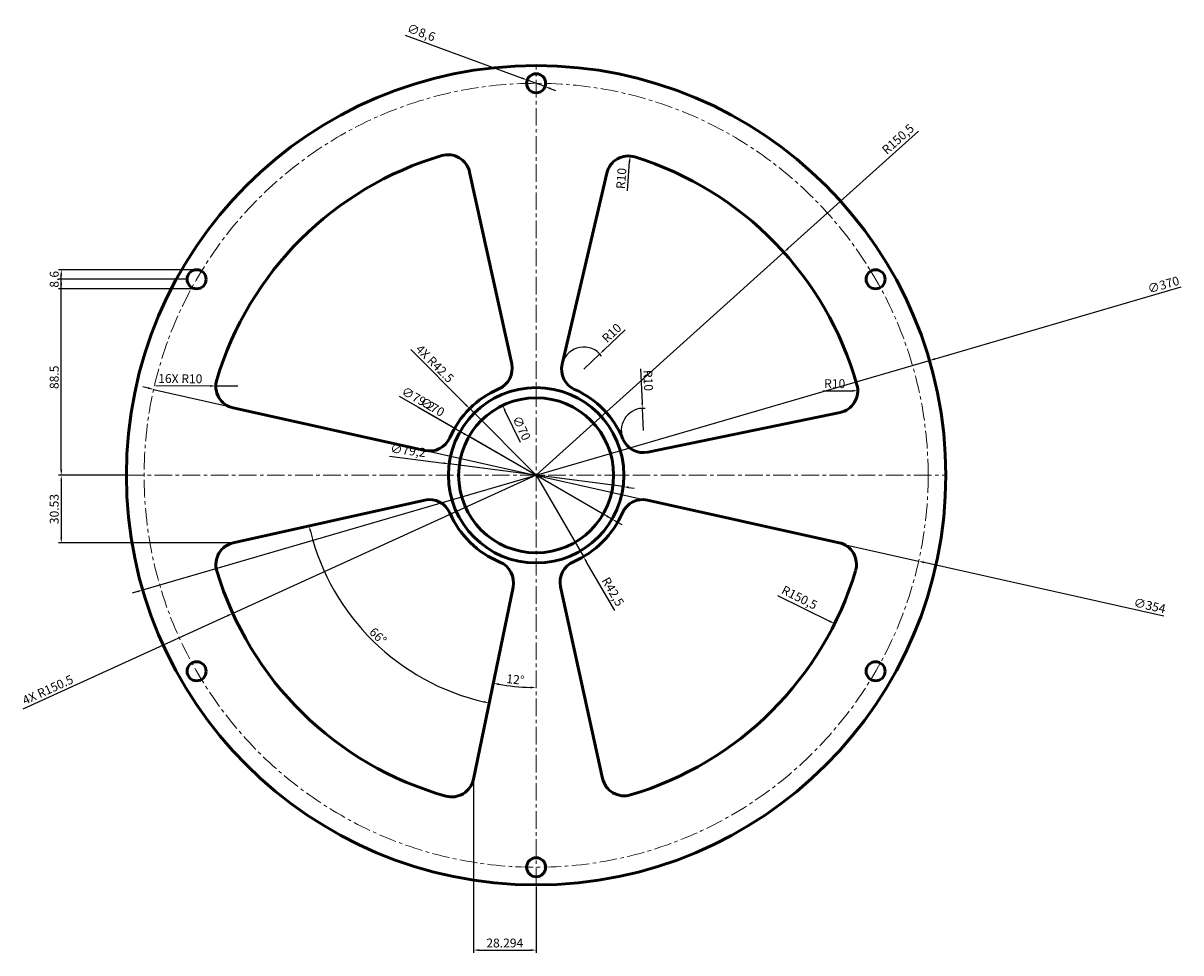
# Model space of a CAD drawing. Units: millimetres. Extents: x 3394 to 3917, y 1441 to 1861.
import ezdxf

# ---------------------------------------------------------------- set-up
doc = ezdxf.new("R2010")
doc.units = ezdxf.units.MM
doc.linetypes.add('CENTER', pattern=[50.8, 31.75, -6.35, 6.35, -6.35])
for name, color, linetype, lineweight in [('M-CNTR', 4, 'CENTER', 18), ('M-DIMS', 2, 'Continuous', 25), ('M-OUTL', 7, 'Continuous', 50)]:
    doc.layers.add(name, color=color, linetype=linetype, lineweight=lineweight)
doc.styles.get("Standard").update_dxf_attribs({"font": 'arial.ttf'})
doc.dimstyles.new('ISO-25', dxfattribs={"dimtxt": 4, "dimasz": 2.5, "dimexe": 1.25, "dimexo": 0.625, "dimtad": 1, "dimtxsty": 'Standard', "dimcen": 4, "dimadec": 0, "dimazin": 0, "dimtfac": 1, "dimtmove": 0, "dimatfit": 3, "dimfxl": 1, "dimarcsym": 0})

# ---------------------------------------------------------------- blocks, each defined once
blk = doc.blocks.new('*U1')
blk.add_circle((0, 0), 4.3)
blk = doc.blocks.new('*U2')
at = {"layer": 'M-OUTL', "color": 0, "linetype": 'ByBlock', "lineweight": -2, "transparency": 16777216}
blk.add_blockref('*U1', (3625.59, 1833.5), dxfattribs=at)
for p, rotation in [((3472.3, 1745), 59.99999999999999), ((3778.87, 1745), 300), ((3472.3, 1568), 120), ((3778.87, 1568), 240), ((3625.59, 1479.5), 180)]:
    blk.add_blockref('*U1', p, dxfattribs=dict(at, rotation=rotation))
blk = doc.blocks.new('*D3')
at = {"layer": 'Defpoints', "color": 0, "transparency": 16777216}
for p in [(3737.44, 1757.19), (3625.59, 1656.5)]:
    blk.add_point(p, dxfattribs=at)
at = {"layer": 'M-DIMS', "color": 0, "lineweight": -2, "transparency": 16777216}
for p, q in [((3798.24, 1811.91), (3739.3, 1758.86)), ((3625.59, 1656.5), (3737.44, 1757.19))]:
    blk.add_line(p, q, dxfattribs=at)
at = {"layer": 'M-DIMS', "color": 0, "transparency": 16777216}
blk.add_solid([(3739.02, 1759.17), (3739.58, 1758.55), (3737.44, 1757.19)], dxfattribs=at)
at = {"layer": 'M-DIMS', "color": 0, "transparency": 16777216, "insert": (3789.3, 1807.94), "char_height": 4, "attachment_point": 5, "rotation": 41.9925}
blk.add_mtext('R150,5', dxfattribs=at)
blk = doc.blocks.new('*D4')
at = {"layer": 'Defpoints', "color": 0, "transparency": 16777216}
for p in [(3654.32, 1711.28), (3647.06, 1704.41)]:
    blk.add_point(p, dxfattribs=at)
at = {"layer": 'M-DIMS', "color": 0, "lineweight": -2, "transparency": 16777216}
for p, q in [((3665.79, 1722.14), (3656.14, 1713)), ((3647.06, 1704.41), (3654.32, 1711.28))]:
    blk.add_line(p, q, dxfattribs=at)
blk.add_arc((3647.06, 1704.41), 10, 36.2819, 163.2566, dxfattribs=at)
at = {"layer": 'M-DIMS', "color": 0, "transparency": 16777216}
blk.add_solid([(3655.85, 1713.31), (3656.42, 1712.7), (3654.32, 1711.28)], dxfattribs=at)
at = {"layer": 'M-DIMS', "color": 0, "transparency": 16777216, "insert": (3660.04, 1720.37), "char_height": 4, "attachment_point": 5, "rotation": 43.4438}
blk.add_mtext('R10', dxfattribs=at)
blk = doc.blocks.new('*D5')
at = {"layer": 'Defpoints', "color": 0, "transparency": 16777216}
for p in [(3667.98, 1800.66), (3667.24, 1790.68)]:
    blk.add_point(p, dxfattribs=at)
at = {"layer": 'M-DIMS', "color": 0, "lineweight": -2, "transparency": 16777216}
blk.add_line((3666.8, 1784.91), (3667.8, 1798.16), dxfattribs=at)
at = {"layer": 'M-DIMS', "color": 0, "transparency": 16777216}
blk.add_solid([(3667.38, 1798.19), (3668.21, 1798.13), (3667.98, 1800.66)], dxfattribs=at)
at = {"layer": 'M-DIMS', "color": 0, "transparency": 16777216, "insert": (3664.55, 1790.49), "char_height": 4, "attachment_point": 5, "rotation": 85.7143}
blk.add_mtext('R10', dxfattribs=at)
blk = doc.blocks.new('*D6')
at = {"layer": 'Defpoints', "color": 0, "transparency": 16777216}
for p in [(3760.8, 1694.67), (3770.8, 1694.67)]:
    blk.add_point(p, dxfattribs=at)
at = {"layer": 'M-DIMS', "color": 0, "lineweight": -2, "transparency": 16777216}
blk.add_line((3755.01, 1694.67), (3768.3, 1694.67), dxfattribs=at)
at = {"layer": 'M-DIMS', "color": 0, "transparency": 16777216}
blk.add_solid([(3768.3, 1695.09), (3768.3, 1694.26), (3770.8, 1694.67)], dxfattribs=at)
at = {"layer": 'M-DIMS', "color": 0, "transparency": 16777216, "insert": (3760.4, 1697.34), "char_height": 4, "attachment_point": 5}
blk.add_mtext('R10', dxfattribs=at)
blk = doc.blocks.new('*D7')
at = {"layer": 'Defpoints', "color": 0, "transparency": 16777216}
for p in [(3673.57, 1686.72), (3674.03, 1676.73)]:
    blk.add_point(p, dxfattribs=at)
at = {"layer": 'M-DIMS', "color": 0, "lineweight": -2, "transparency": 16777216}
for p, q in [((3672.74, 1704.56), (3673.45, 1689.22)), ((3674.03, 1676.73), (3673.57, 1686.72))]:
    blk.add_line(p, q, dxfattribs=at)
blk.add_arc((3674.03, 1676.73), 10, 85.5012, 199.0838, dxfattribs=at)
at = {"layer": 'M-DIMS', "color": 0, "transparency": 16777216}
blk.add_solid([(3673.87, 1689.24), (3673.04, 1689.2), (3673.57, 1686.72)], dxfattribs=at)
at = {"layer": 'M-DIMS', "color": 0, "transparency": 16777216, "insert": (3675.65, 1699.29), "char_height": 4, "attachment_point": 5, "rotation": 272.6632}
blk.add_mtext('R10', dxfattribs=at)
blk = doc.blocks.new('*D8')
at = {"layer": 'Defpoints', "color": 0, "transparency": 16777216}
for p in [(3625.59, 1656.5), (3646.96, 1619.76)]:
    blk.add_point(p, dxfattribs=at)
at = {"layer": 'M-DIMS', "color": 0, "lineweight": -2, "transparency": 16777216}
for p, q in [((3625.59, 1656.5), (3646.96, 1619.76)), ((3661.09, 1595.47), (3648.22, 1617.6))]:
    blk.add_line(p, q, dxfattribs=at)
at = {"layer": 'M-DIMS', "color": 0, "transparency": 16777216}
blk.add_solid([(3648.58, 1617.81), (3647.86, 1617.39), (3646.96, 1619.76)], dxfattribs=at)
at = {"layer": 'M-DIMS', "color": 0, "transparency": 16777216, "insert": (3659.81, 1603.69), "char_height": 4, "attachment_point": 5, "rotation": 300.1914}
blk.add_mtext('R42,5', dxfattribs=at)
blk = doc.blocks.new('*D9')
at = {"layer": 'Defpoints', "color": 0, "transparency": 16777216}
for p in [(3625.59, 1656.5), (3760.34, 1589.48)]:
    blk.add_point(p, dxfattribs=at)
at = {"layer": 'M-DIMS', "color": 0, "lineweight": -2, "transparency": 16777216}
blk.add_line((3734.59, 1602.28), (3758.1, 1590.59), dxfattribs=at)
at = {"layer": 'M-DIMS', "color": 0, "transparency": 16777216}
blk.add_solid([(3758.29, 1590.96), (3757.91, 1590.22), (3760.34, 1589.48)], dxfattribs=at)
at = {"layer": 'M-DIMS', "color": 0, "transparency": 16777216, "insert": (3744.27, 1600.85), "char_height": 4, "attachment_point": 5, "rotation": 333.555}
blk.add_mtext('R150,5', dxfattribs=at)
blk = doc.blocks.new('*D10')
at = {"layer": 'Defpoints', "color": 0, "transparency": 16777216}
for p in [(3621.55, 1834.98), (3629.62, 1832.01)]:
    blk.add_point(p, dxfattribs=at)
at = {"layer": 'M-DIMS', "color": 0, "lineweight": -2, "transparency": 16777216}
for p, q in [((3566.44, 1855.27), (3619.21, 1835.85)), ((3629.62, 1832.01), (3621.55, 1834.98)), ((3631.97, 1831.15), (3634.31, 1830.29))]:
    blk.add_line(p, q, dxfattribs=at)
at = {"layer": 'M-DIMS', "color": 0, "transparency": 16777216}
for points in [[(3619.35, 1836.24), (3619.06, 1835.46), (3621.55, 1834.98)], [(3632.11, 1831.54), (3631.82, 1830.76), (3629.62, 1832.01)]]:
    blk.add_solid(points, dxfattribs=at)
at = {"layer": 'M-DIMS', "color": 0, "transparency": 16777216, "insert": (3573.55, 1855.95), "char_height": 4, "attachment_point": 5, "rotation": 339.7938}
blk.add_mtext('∅8,6', dxfattribs=at)
blk = doc.blocks.new('*D11')
at = {"layer": 'Defpoints', "color": 0, "transparency": 16777216}
for p in [(3586.32, 1661.63), (3664.85, 1651.37)]:
    blk.add_point(p, dxfattribs=at)
at = {"layer": 'M-DIMS', "color": 0, "lineweight": -2, "transparency": 16777216}
for p, q in [((3559.41, 1665.15), (3583.84, 1661.96)), ((3664.85, 1651.37), (3586.32, 1661.63)), ((3667.33, 1651.04), (3669.81, 1650.72))]:
    blk.add_line(p, q, dxfattribs=at)
at = {"layer": 'M-DIMS', "color": 0, "transparency": 16777216}
for points in [[(3583.9, 1662.37), (3583.79, 1661.54), (3586.32, 1661.63)], [(3667.39, 1651.46), (3667.28, 1650.63), (3664.85, 1651.37)]]:
    blk.add_solid(points, dxfattribs=at)
at = {"layer": 'M-DIMS', "color": 0, "transparency": 16777216, "insert": (3567.72, 1667.18), "char_height": 4, "attachment_point": 5, "rotation": 352.5521}
blk.add_mtext('∅79,2', dxfattribs=at)
blk = doc.blocks.new('*D12')
at = {"layer": 'Defpoints', "color": 0, "transparency": 16777216}
for p in [(3610.45, 1688.06), (3640.72, 1624.94)]:
    blk.add_point(p, dxfattribs=at)
at = {"layer": 'M-DIMS', "color": 0, "lineweight": -2, "transparency": 16777216}
blk.add_line((3618.5, 1671.28), (3611.53, 1685.8), dxfattribs=at)
at = {"layer": 'M-DIMS', "color": 0, "transparency": 16777216}
blk.add_solid([(3611.91, 1685.98), (3611.16, 1685.62), (3610.45, 1688.06)], dxfattribs=at)
at = {"layer": 'M-DIMS', "color": 0, "transparency": 16777216, "insert": (3618.55, 1677.59), "char_height": 4, "attachment_point": 5, "rotation": 295.6238}
blk.add_mtext('∅70', dxfattribs=at)
blk = doc.blocks.new('*D13')
at = {"layer": 'Defpoints', "color": 0, "transparency": 16777216}
for p in [(3575.29, 1645.27), (3488.81, 1625.97), (3615.18, 1606.02), (3539.07, 1597.03), (3597.29, 1519.24)]:
    blk.add_point(p, dxfattribs=at)
at = {"layer": 'M-DIMS', "color": 0, "lineweight": -2, "transparency": 16777216}
blk.add_arc((3625.59, 1656.5), 104.99, 193.9465, 256.9878, dxfattribs=at)
at = {"layer": 'M-DIMS', "color": 0, "transparency": 16777216}
for points in [[(3523.29, 1631.1), (3524.1, 1631.29), (3523.12, 1633.63)], [(3602.04, 1554.62), (3601.86, 1553.8), (3604.39, 1553.67)]]:
    blk.add_solid(points, dxfattribs=at)
at = {"layer": 'M-DIMS', "color": 0, "transparency": 16777216, "insert": (3553.83, 1583.56), "char_height": 4, "attachment_point": 5, "rotation": 315.4671}
blk.add_mtext('66°', dxfattribs=at)
blk = doc.blocks.new('*D14')
at = {"layer": 'Defpoints', "color": 0, "transparency": 16777216}
for p in [(3625.59, 1841.5), (3615.18, 1606.02), (3612.64, 1561.54), (3597.29, 1519.24), (3625.59, 1471.5)]:
    blk.add_point(p, dxfattribs=at)
at = {"layer": 'M-DIMS', "color": 0, "lineweight": -2, "transparency": 16777216}
blk.add_arc((3625.59, 1656.5), 95.84, 259.8467, 268.5054, dxfattribs=at)
at = {"layer": 'M-DIMS', "color": 0, "transparency": 16777216}
for points in [[(3608.61, 1561.75), (3608.77, 1562.57), (3606.24, 1562.63)], [(3623.09, 1561.11), (3623.08, 1560.27), (3625.59, 1560.66)]]:
    blk.add_solid(points, dxfattribs=at)
at = {"layer": 'M-DIMS', "color": 0, "transparency": 16777216, "insert": (3616.13, 1563.77), "char_height": 4, "attachment_point": 5, "rotation": 354.1761}
blk.add_mtext('12°', dxfattribs=at)
blk = doc.blocks.new('DISC-CUTOUT')
for p, q in [((133.58, 39.38), (114.6, 125.93)), ((94.31, 0.24), (7.83, 19.49))]:
    blk.add_line(p, q)
for centre, radius, start, end in [((144.62, -10.96), 150.5, 106.4509, 163.3683), ((104.83, 123.79), 10, 12.3694, 106.4509), ((123.81, 37.24), 10, 293.35, 12.3694), ((10, 29.25), 10, 163.3683, 257.4497), ((144.62, -10.96), 42.5, 113.35, 156.4691), ((96.49, 10), 10, 257.4497, 336.4691)]:
    blk.add_arc(centre, radius, start, end)
blk = doc.blocks.new('*D16')
at = {"layer": 'Defpoints', "color": 0, "transparency": 16777216}
for p in [(3411.19, 1749.3), (3472.3, 1749.3), (3472.3, 1740.7)]:
    blk.add_point(p, dxfattribs=at)
at = {"layer": 'M-DIMS', "color": 0, "lineweight": -2, "transparency": 16777216}
for p, q in [((3471.68, 1749.3), (3409.94, 1749.3)), ((3411.19, 1743.2), (3411.19, 1746.8)), ((3471.68, 1740.7), (3409.94, 1740.7))]:
    blk.add_line(p, q, dxfattribs=at)
at = {"layer": 'M-DIMS', "color": 0, "transparency": 16777216}
for points in [[(3410.77, 1746.8), (3411.6, 1746.8), (3411.19, 1749.3)], [(3410.77, 1743.2), (3411.6, 1743.2), (3411.19, 1740.7)]]:
    blk.add_solid(points, dxfattribs=at)
at = {"layer": 'M-DIMS', "color": 0, "transparency": 16777216, "insert": (3408.52, 1745), "char_height": 4, "attachment_point": 5, "rotation": 90}
blk.add_mtext('8.6', dxfattribs=at)
blk = doc.blocks.new('*D17')
at = {"layer": 'Defpoints', "color": 0, "transparency": 16777216}
for p in [(3411.19, 1745), (3468, 1745), (3440.59, 1656.5)]:
    blk.add_point(p, dxfattribs=at)
at = {"layer": 'M-DIMS', "color": 0, "lineweight": -2, "transparency": 16777216}
for p, q in [((3467.38, 1745), (3409.94, 1745)), ((3411.19, 1659), (3411.19, 1742.5)), ((3439.96, 1656.5), (3409.94, 1656.5))]:
    blk.add_line(p, q, dxfattribs=at)
at = {"layer": 'M-DIMS', "color": 0, "transparency": 16777216}
for points in [[(3410.77, 1742.5), (3411.6, 1742.5), (3411.19, 1745)], [(3410.77, 1659), (3411.6, 1659), (3411.19, 1656.5)]]:
    blk.add_solid(points, dxfattribs=at)
at = {"layer": 'M-DIMS', "color": 0, "transparency": 16777216, "insert": (3408.52, 1700.75), "char_height": 4, "attachment_point": 5, "rotation": 90}
blk.add_mtext('88.5', dxfattribs=at)
blk = doc.blocks.new('*D18')
at = {"layer": 'Defpoints', "color": 0, "transparency": 16777216}
for p in [(3597.29, 1519.24), (3625.59, 1471.5), (3625.59, 1442.1)]:
    blk.add_point(p, dxfattribs=at)
at = {"layer": 'M-DIMS', "color": 0, "lineweight": -2, "transparency": 16777216}
for p, q in [((3597.29, 1518.62), (3597.29, 1440.85)), ((3625.59, 1470.87), (3625.59, 1440.85)), ((3599.79, 1442.1), (3623.09, 1442.1))]:
    blk.add_line(p, q, dxfattribs=at)
at = {"layer": 'M-DIMS', "color": 0, "transparency": 16777216}
for points in [[(3599.79, 1442.52), (3599.79, 1441.68), (3597.29, 1442.1)], [(3623.09, 1442.52), (3623.09, 1441.68), (3625.59, 1442.1)]]:
    blk.add_solid(points, dxfattribs=at)
at = {"layer": 'M-DIMS', "color": 0, "transparency": 16777216, "insert": (3611.44, 1444.77), "char_height": 4, "attachment_point": 5}
blk.add_mtext('28.294', dxfattribs=at)
blk = doc.blocks.new('*D19')
at = {"layer": 'Defpoints', "color": 0, "transparency": 16777216}
for p in [(3440.59, 1656.5), (3411.19, 1625.97), (3488.81, 1625.97)]:
    blk.add_point(p, dxfattribs=at)
at = {"layer": 'M-DIMS', "color": 0, "lineweight": -2, "transparency": 16777216}
for p, q in [((3439.96, 1656.5), (3409.94, 1656.5)), ((3411.19, 1654), (3411.19, 1628.47)), ((3488.18, 1625.97), (3409.94, 1625.97))]:
    blk.add_line(p, q, dxfattribs=at)
at = {"layer": 'M-DIMS', "color": 0, "transparency": 16777216}
for points in [[(3410.77, 1654), (3411.6, 1654), (3411.19, 1656.5)], [(3410.77, 1628.47), (3411.6, 1628.47), (3411.19, 1625.97)]]:
    blk.add_solid(points, dxfattribs=at)
at = {"layer": 'M-DIMS', "color": 0, "transparency": 16777216, "insert": (3408.52, 1641.24), "char_height": 4, "attachment_point": 5, "rotation": 90}
blk.add_mtext('30.53', dxfattribs=at)
blk = doc.blocks.new('*D20')
at = {"layer": 'Defpoints', "color": 0, "transparency": 16777216}
for p in [(3591.29, 1676.3), (3659.88, 1636.7)]:
    blk.add_point(p, dxfattribs=at)
at = {"layer": 'M-DIMS', "color": 0, "lineweight": -2, "transparency": 16777216}
for p, q in [((3563.81, 1692.16), (3589.13, 1677.55)), ((3659.88, 1636.7), (3591.29, 1676.3)), ((3662.05, 1635.45), (3664.21, 1634.2))]:
    blk.add_line(p, q, dxfattribs=at)
at = {"layer": 'M-DIMS', "color": 0, "transparency": 16777216}
for points in [[(3589.33, 1677.91), (3588.92, 1677.19), (3591.29, 1676.3)], [(3662.26, 1635.81), (3661.84, 1635.09), (3659.88, 1636.7)]]:
    blk.add_solid(points, dxfattribs=at)
at = {"layer": 'M-DIMS', "color": 0, "transparency": 16777216, "insert": (3572.1, 1690.58), "char_height": 4, "attachment_point": 5, "rotation": 330.0029}
blk.add_mtext('∅79.2', dxfattribs=at)
blk = doc.blocks.new('*D21')
at = {"layer": 'Defpoints', "color": 0, "transparency": 16777216}
for p in [(3803.19, 1708.3), (3447.99, 1604.7)]:
    blk.add_point(p, dxfattribs=at)
at = {"layer": 'M-DIMS', "color": 0, "lineweight": -2, "transparency": 16777216}
for p, q in [((3916.67, 1741.4), (3805.59, 1709)), ((3447.99, 1604.7), (3803.19, 1708.3)), ((3445.59, 1604), (3443.19, 1603.3))]:
    blk.add_line(p, q, dxfattribs=at)
at = {"layer": 'M-DIMS', "color": 0, "transparency": 16777216}
for points in [[(3805.47, 1709.4), (3805.7, 1708.6), (3803.19, 1708.3)], [(3445.47, 1604.4), (3445.7, 1603.6), (3447.99, 1604.7)]]:
    blk.add_solid(points, dxfattribs=at)
at = {"layer": 'M-DIMS', "color": 0, "transparency": 16777216, "insert": (3908.97, 1742.05), "char_height": 4, "attachment_point": 5, "rotation": 16.2601}
blk.add_mtext('∅370', dxfattribs=at)
blk = doc.blocks.new('*D22')
at = {"layer": 'Defpoints', "color": 0, "transparency": 16777216}
for p in [(3452.89, 1695.3), (3798.28, 1617.7)]:
    blk.add_point(p, dxfattribs=at)
at = {"layer": 'M-DIMS', "color": 0, "lineweight": -2, "transparency": 16777216}
for p, q in [((3450.45, 1695.85), (3448.01, 1696.4)), ((3452.89, 1695.3), (3798.28, 1617.7)), ((3908.93, 1592.84), (3800.72, 1617.15))]:
    blk.add_line(p, q, dxfattribs=at)
at = {"layer": 'M-DIMS', "color": 0, "transparency": 16777216}
for points in [[(3450.54, 1696.25), (3450.36, 1695.44), (3452.89, 1695.3)], [(3800.81, 1617.56), (3800.63, 1616.75), (3798.28, 1617.7)]]:
    blk.add_solid(points, dxfattribs=at)
at = {"layer": 'M-DIMS', "color": 0, "transparency": 16777216, "insert": (3902.51, 1597.13), "char_height": 4, "attachment_point": 5, "rotation": 347.3375}
blk.add_mtext('∅354', dxfattribs=at)
blk = doc.blocks.new('*D23')
at = {"layer": 'Defpoints', "color": 0, "transparency": 16777216}
for p in [(3625.59, 1656.5), (3488.61, 1594.15)]:
    blk.add_point(p, dxfattribs=at)
at = {"layer": 'M-DIMS', "color": 0, "lineweight": -2, "transparency": 16777216}
for p, q in [((3625.59, 1656.5), (3488.61, 1594.15)), ((3393.97, 1551.07), (3486.33, 1593.11))]:
    blk.add_line(p, q, dxfattribs=at)
at = {"layer": 'M-DIMS', "color": 0, "transparency": 16777216}
blk.add_solid([(3486.16, 1593.49), (3486.51, 1592.73), (3488.61, 1594.15)], dxfattribs=at)
at = {"layer": 'M-DIMS', "color": 0, "transparency": 16777216, "insert": (3405.32, 1559.17), "char_height": 4, "attachment_point": 5, "rotation": 24.4742}
blk.add_mtext('4X R150.5', dxfattribs=at)
blk = doc.blocks.new('*D24')
at = {"layer": 'Defpoints', "color": 0, "transparency": 16777216}
for p in [(3595.58, 1686.6), (3625.59, 1656.5)]:
    blk.add_point(p, dxfattribs=at)
at = {"layer": 'M-DIMS', "color": 0, "lineweight": -2, "transparency": 16777216}
for p, q in [((3569.02, 1713.25), (3593.82, 1688.37)), ((3625.59, 1656.5), (3595.58, 1686.6))]:
    blk.add_line(p, q, dxfattribs=at)
at = {"layer": 'M-DIMS', "color": 0, "transparency": 16777216}
blk.add_solid([(3594.11, 1688.66), (3593.52, 1688.08), (3595.58, 1686.6)], dxfattribs=at)
at = {"layer": 'M-DIMS', "color": 0, "transparency": 16777216, "insert": (3579.47, 1706.54), "char_height": 4, "attachment_point": 5, "rotation": 314.9094}
blk.add_mtext('4X R42.5', dxfattribs=at)
blk = doc.blocks.new('*D25')
at = {"layer": 'Defpoints', "color": 0, "transparency": 16777216}
for p in [(3595.28, 1674), (3655.9, 1639)]:
    blk.add_point(p, dxfattribs=at)
at = {"layer": 'M-DIMS', "color": 0, "lineweight": -2, "transparency": 16777216}
for p, q in [((3572.19, 1687.33), (3593.11, 1675.25)), ((3655.9, 1639), (3595.28, 1674)), ((3658.06, 1637.75), (3660.23, 1636.5))]:
    blk.add_line(p, q, dxfattribs=at)
at = {"layer": 'M-DIMS', "color": 0, "transparency": 16777216}
for points in [[(3593.32, 1675.61), (3592.9, 1674.89), (3595.28, 1674)], [(3658.27, 1638.11), (3657.85, 1637.39), (3655.9, 1639)]]:
    blk.add_solid(points, dxfattribs=at)
at = {"layer": 'M-DIMS', "color": 0, "transparency": 16777216, "insert": (3578.48, 1686.91), "char_height": 4, "attachment_point": 5, "rotation": 329.9957}
blk.add_mtext('∅70', dxfattribs=at)
blk = doc.blocks.new('*D26')
at = {"layer": 'Defpoints', "color": 0, "transparency": 16777216}
for p in [(3480.96, 1696.8), (3490.96, 1696.71)]:
    blk.add_point(p, dxfattribs=at)
at = {"layer": 'M-DIMS', "color": 0, "lineweight": -2, "transparency": 16777216}
for p, q in [((3453.85, 1697.04), (3478.46, 1696.82)), ((3490.96, 1696.71), (3480.96, 1696.8))]:
    blk.add_line(p, q, dxfattribs=at)
at = {"layer": 'M-DIMS', "color": 0, "transparency": 16777216}
blk.add_solid([(3478.47, 1697.24), (3478.46, 1696.41), (3480.96, 1696.8)], dxfattribs=at)
at = {"layer": 'M-DIMS', "color": 0, "transparency": 16777216, "insert": (3464.93, 1699.61), "char_height": 4, "attachment_point": 5, "rotation": 359.5006}
blk.add_mtext('16X R10', dxfattribs=at)

msp = doc.modelspace()

# ---------------------------------------------------------------- linework, layer by layer
at = {"layer": 'M-CNTR', "ltscale": 0.25, "transparency": 33554534}
for p, q in [((3625.5865, 1471.4995), (3625.5865, 1841.4995)), ((3440.5865, 1656.4995), (3810.5865, 1656.4995))]:
    msp.add_line(p, q, dxfattribs=at)
msp.add_circle((3625.5865, 1656.4995), 177, dxfattribs=at)
at = {"layer": 'M-OUTL'}
for p, q in [((3637.3225, 1706.6843), (3657.4989, 1792.9614)), ((3676.0574, 1666.937), (3762.8262, 1684.8809)), ((3575.2854, 1645.2723), (3488.8084, 1625.9707)), ((3615.181, 1606.022), (3597.2921, 1519.2418))]:
    msp.add_line(p, q, dxfattribs=at)
for radius in [185, 39.6, 35]:
    msp.add_circle((3625.5865, 1656.4995), radius, dxfattribs=at)
for centre, radius, start, end in [((3667.2362, 1790.6842), 10, 72.756141, 166.837583), ((3625.5865, 1656.4995), 150.5, 15.765631, 72.756141), ((3647.0598, 1704.4072), 10, 166.837583, 245.857008), ((3625.5865, 1656.4995), 42.5, 22.664764, 65.857008), ((3760.8011, 1694.6737), 10, 281.684189, 15.765631), ((3674.0322, 1676.7297), 10, 202.664764, 281.684189), ((3577.4638, 1635.5124), 10, 23.562718, 102.582142), ((3625.5865, 1656.4995), 42.5, 203.562718, 247.371573), ((3490.9868, 1616.2108), 10, 102.582142, 196.663585), ((3605.387, 1608.0409), 10, 348.352148, 67.371573), ((3625.5865, 1656.4995), 150.5, 196.663585, 254.270706), ((3587.498, 1521.2607), 10, 254.270706, 348.352148)]:
    msp.add_arc(centre, radius, start, end, dxfattribs=at)

# ---------------------------------------------------------------- block references
for name, p in [('*U2', (0, 0)), ('DISC-CUTOUT', (3480.966, 1667.459))]:
    msp.add_blockref(name, p, dxfattribs=at)
at = {"layer": 'M-OUTL', "rotation": 180}
msp.add_blockref('DISC-CUTOUT', (3770.207, 1645.5399), dxfattribs=at)

# ---------------------------------------------------------------- dimensions: what is measured, and where the dimension line sits
at = {"layer": 'M-DIMS'}
for p1, p2, override, picture, middle in [((3629.6219, 1832.0142), (3621.5512, 1834.9847), {"dimclrd": 0, "dimclre": 0, "dimclrt": 0}, '*D10', (3572.4824, 1853.0445)), ((3447.9864, 1604.6999), (3803.1866, 1708.299), {"dimdec": 0, "dimlfac": 1, "dimrnd": 0, "dimzin": 0, "dimdsep": 46, "dimlunit": 2}, '*D21', (3909.7467, 1739.3788)), ((3452.8915, 1695.2993), (3798.2815, 1617.6997), {"dimdec": 0, "dimlfac": 1, "dimrnd": 0, "dimzin": 0, "dimdsep": 46, "dimlunit": 2}, '*D22', (3901.8986, 1594.4198)), ((3659.8821, 1636.7012), (3591.2909, 1676.2977), {"dimdec": 1, "dimlfac": 1, "dimrnd": 0, "dimzin": 0, "dimdsep": 46, "dimlunit": 2}, '*D20', (3570.7135, 1688.1767)), ((3655.8961, 1638.9972), (3595.277, 1674.0018), {"dimdec": 0, "dimlfac": 1, "dimrnd": 0, "dimzin": 0, "dimdsep": 46, "dimlunit": 2}, '*D25', (3577.0912, 1684.5031)), ((3640.7226, 1624.9416), (3610.4504, 1688.0573), {"dimclrd": 0, "dimclre": 0, "dimclrt": 0}, '*D12', (3616.0481, 1676.3864)), ((3664.8524, 1651.3663), (3586.3206, 1661.6326), {"dimclrd": 0, "dimclre": 0, "dimclrt": 0}, '*D11', (3567.3186, 1664.1167))]:
    dim = msp.add_diameter_dim_2p(p1=p1, p2=p2, dimstyle='ISO-25', override=override, dxfattribs=at)
    dim.commit()
    dim.dimension.update_dxf_attribs({"geometry": picture, "text_midpoint": middle, "dimtype": 163})
for base, line1, line2, picture, middle in [((3612.637, 1561.5371), ((3615.181, 1606.022), (3597.2921, 1519.2418)), ((3625.5865, 1471.4995), (3625.5865, 1841.4995)), '*D14', (3616.1285, 1563.7725)), ((3539.0698, 1597.026), ((3575.2854, 1645.2723), (3488.8084, 1625.9707)), ((3615.181, 1606.022), (3597.2921, 1519.2418)), '*D13', (3553.8279, 1583.5611))]:
    dim = msp.add_angular_dim_2l(base=base, line1=line1, line2=line2, dimstyle='ISO-25', override={"dimclrd": 0, "dimclre": 0, "dimclrt": 0}, dxfattribs=at)
    dim.commit()
    dim.dimension.update_dxf_attribs({"geometry": picture, "text_midpoint": middle})
for center, mpoint, picture, middle in [((3625.5865, 1656.4995), (3737.443, 1757.189), '*D3', (3791.3239, 1805.6909)), ((3667.2362, 1790.6842), (3667.9835, 1800.6563), '*D5', (3667.2065, 1790.2882)), ((3674.0322, 1676.7297), (3673.5676, 1686.7189), '*D7', (3672.9884, 1699.1691)), ((3760.8011, 1694.6737), (3770.8011, 1694.6737), '*D6', (3760.4039, 1694.6737)), ((3625.5865, 1656.4995), (3646.9594, 1619.7646), '*D8', (3657.1952, 1602.1715)), ((3625.5865, 1656.4995), (3760.3385, 1589.476), '*D9', (3742.9166, 1598.1414))]:
    dim = msp.add_radius_dim(center=center, mpoint=mpoint, dimstyle='ISO-25', override={"dimclrd": 0, "dimclre": 0, "dimclrt": 0}, dxfattribs=at)
    dim.commit()
    dim.dimension.update_dxf_attribs({"geometry": picture, "text_midpoint": middle, "dimtype": 164})
for base, p1, p2, override, picture, middle in [((3411.1865, 1749.2995), (3472.3, 1740.6995), (3472.3, 1749.2995), {"dimdec": 1, "dimlfac": 1, "dimrnd": 0, "dimzin": 0, "dimdsep": 46, "dimlunit": 2}, '*D16', (3408.5192, 1744.9995)), ((3411.1865, 1744.9995), (3440.5865, 1656.4995), (3468, 1744.9995), {"dimdec": 1, "dimlfac": 1, "dimrnd": 0, "dimzin": 0, "dimdsep": 46, "dimlunit": 2}, '*D17', (3408.5192, 1700.7495)), ((3411.1865, 1625.9707), (3440.5865, 1656.4995), (3488.8084, 1625.9707), {"dimdec": 2, "dimlfac": 1, "dimrnd": 0, "dimzin": 0, "dimdsep": 46, "dimlunit": 2}, '*D19', (3408.5179, 1641.2351))]:
    dim = msp.add_linear_dim(base=base, p1=p1, p2=p2, angle=90, dimstyle='ISO-25', override=override, dxfattribs=at)
    dim.commit()
    dim.dimension.update_dxf_attribs({"geometry": picture, "text_midpoint": middle})
dim = msp.add_radius_dim(center=(3647.0598, 1704.4072), mpoint=(3654.3203, 1711.2836), dimstyle='ISO-25', override={"dimclrd": 0, "dimclre": 0, "dimclrt": 0}, dxfattribs=at)
dim.commit()
dim.dimension.update_dxf_attribs({"geometry": '*D4', "text_midpoint": (3660.035, 1720.3697)})
for mpoint, picture, middle in [((3595.582, 1686.599), '*D24', (3577.5793, 1704.6587)), ((3488.6093, 1594.1497), '*D23', (3406.4229, 1556.7399))]:
    dim = msp.add_radius_dim(center=(3625.5865, 1656.4995), mpoint=mpoint, text='4X <>', dimstyle='ISO-25', override={"dimdec": 1, "dimlfac": 1, "dimrnd": 0, "dimzin": 0, "dimdsep": 46, "dimlunit": 2}, dxfattribs=at)
    dim.commit()
    dim.dimension.update_dxf_attribs({"geometry": picture, "text_midpoint": middle, "dimtype": 164})
dim = msp.add_radius_dim(center=(3490.9644, 1696.7132), mpoint=(3480.9648, 1696.8004), text='16X <>', dimstyle='ISO-25', override={"dimdec": 0, "dimlfac": 1, "dimrnd": 0, "dimzin": 0, "dimdsep": 46, "dimlunit": 2}, dxfattribs=at)
dim.commit()
dim.dimension.update_dxf_attribs({"geometry": '*D26', "text_midpoint": (3464.9285, 1699.6076)})
dim = msp.add_linear_dim(base=(3625.5865, 1442.0995), p1=(3597.2921, 1519.2418), p2=(3625.5865, 1471.4995), dimstyle='ISO-25', override={"dimdec": 3, "dimlfac": 1, "dimrnd": 0, "dimzin": 0, "dimdsep": 46, "dimlunit": 2}, dxfattribs=at)
dim.commit()
dim.dimension.update_dxf_attribs({"geometry": '*D18', "text_midpoint": (3611.4393, 1444.7668)})

doc.saveas('drawing.dxf')
